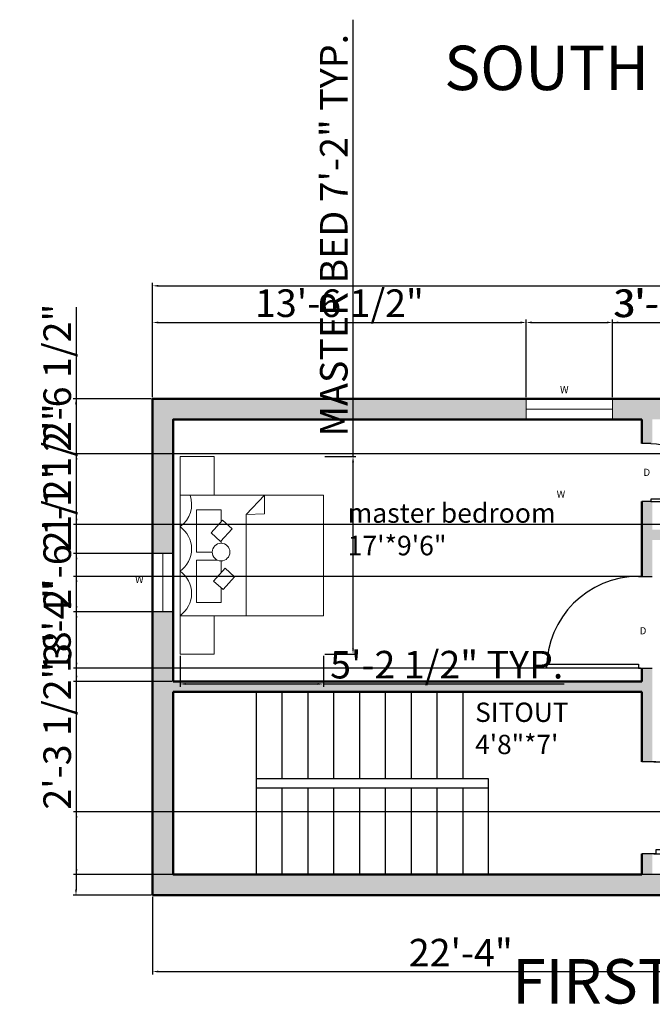
# Model space of a CAD drawing. Units: inches. Extents: x 2225 to 3094, y 1739 to 2599.
# Tile 2 of 5: x 2225 to 2500, y 2171 to 2599. Entities that reach past the tile are written whole.
import ezdxf

# ---------------------------------------------------------------- set-up
doc = ezdxf.new("R2010")
doc.units = ezdxf.units.IN
for name, color, linetype, lineweight in [('A-ANNO-DIMS', 2, 'Continuous', 18), ('A-ANNO-TEXT', 7, 'Continuous', 18), ('A-ANNO-TITL', 7, 'Continuous', 35), ('A-AREA-IDEN', 7, 'Continuous', 18), ('A-DOOR', 4, 'Continuous', 25), ('A-FLOR-STRS', 7, 'Continuous', 25), ('A-FURN', 8, 'Continuous', 18), ('A-WALL-PATT', 160, 'Continuous', 13), ('WALL', 7, 'Continuous', 50), ('WINDOW', 130, 'Continuous', 18)]:
    doc.layers.add(name, color=color, linetype=linetype, lineweight=lineweight)
doc.styles.get("Standard").update_dxf_attribs({"font": 'arial.ttf'})
doc.dimstyles.new('ISO-25', dxfattribs={"dimtxt": 12, "dimasz": 2.5, "dimexe": 1.25, "dimexo": 0.625, "dimtad": 1, "dimdec": 0, "dimlunit": 4, "dimtxsty": 'Standard', "dimcen": 2.5, "dimadec": 0, "dimazin": 0, "dimtfac": 1, "dimtdec": 0, "dimtmove": 0, "dimatfit": 3, "dimfxl": 1, "dimarcsym": 0})

# ---------------------------------------------------------------- blocks, each defined once
blk = doc.blocks.new('*U4')
for p, q in [((0, 0), (0, -6)), ((40, 0), (40, -6))]:
    blk.add_line(p, q)
blk.add_lwpolyline([(0, 0), (0, 40), (1.75, 40), (1.75, 0)], close=True)
blk.add_arc((0, 0), 40, 0, 90)
blk = doc.blocks.new('*D5')
at = {"layer": 'A-ANNO-DIMS', "color": 0, "lineweight": -2, "transparency": 16777216}
for p, q in [((2282.56, 2434.95), (2282.56, 2484.67)), ((2906.56, 2434.95), (2906.56, 2484.67)), ((2285.06, 2483.42), (2904.06, 2483.42))]:
    blk.add_line(p, q, dxfattribs=at)
at = {"layer": 'A-ANNO-DIMS', "color": 0, "transparency": 16777216}
for points in [[(2285.06, 2483.83), (2285.06, 2483), (2282.56, 2483.42)], [(2904.06, 2483.83), (2904.06, 2483), (2906.56, 2483.42)]]:
    blk.add_solid(points, dxfattribs=at)
at = {"layer": 'Defpoints', "color": 0, "transparency": 16777216}
for p in [(2906.56, 2483.42), (2282.56, 2434.33), (2906.56, 2434.33)]:
    blk.add_point(p, dxfattribs=at)
at = {"layer": 'A-ANNO-DIMS', "color": 0, "transparency": 16777216, "insert": (2594.56, 2490.17), "char_height": 12, "attachment_point": 5}
blk.add_mtext("52'", dxfattribs=at)
blk = doc.blocks.new('*D6')
at = {"layer": 'A-ANNO-DIMS', "color": 0, "lineweight": -2, "transparency": 16777216}
for p, q in [((2281.93, 2434.33), (2247.95, 2434.33)), ((2249.2, 2431.83), (2249.2, 2220.83)), ((2281.93, 2218.33), (2247.95, 2218.33))]:
    blk.add_line(p, q, dxfattribs=at)
at = {"layer": 'A-ANNO-DIMS', "color": 0, "transparency": 16777216}
for points in [[(2248.78, 2431.83), (2249.61, 2431.83), (2249.2, 2434.33)], [(2248.78, 2220.83), (2249.61, 2220.83), (2249.2, 2218.33)]]:
    blk.add_solid(points, dxfattribs=at)
at = {"layer": 'Defpoints', "color": 0, "transparency": 16777216}
for p in [(2282.56, 2434.33), (2249.2, 2218.33), (2282.56, 2218.33)]:
    blk.add_point(p, dxfattribs=at)
at = {"layer": 'A-ANNO-DIMS', "color": 0, "transparency": 16777216, "insert": (2242.45, 2326.33), "char_height": 12, "attachment_point": 5, "rotation": 90}
blk.add_mtext("18'", dxfattribs=at)
blk = doc.blocks.new('STAIR-RETURN')
for p, q in [((0, 79.5), (36, 79.5)), ((36, 79.5), (36, 0)), ((47.27, 79.5), (47.27, 41.75)), ((58.52, 79.5), (58.52, 41.75)), ((69.77, 79.5), (69.77, 41.75)), ((81.01, 79.5), (81.01, 41.75)), ((92.26, 79.5), (92.26, 41.75)), ((103.51, 79.5), (103.51, 41.75)), ((114.75, 79.5), (114.75, 41.75)), ((204, 79.5), (126, 79.5)), ((126, 79.5), (126, 41.75)), ((36, 41.75), (126, 41.75)), ((126, 41.75), (137, 41.75)), ((137, 41.75), (137, 0)), ((36, 37.75), (126, 37.75)), ((47.27, 37.75), (47.27, 0)), ((58.52, 37.75), (58.52, 0)), ((69.77, 37.75), (69.77, 0)), ((81.01, 37.75), (81.01, 0)), ((92.26, 37.75), (92.26, 0)), ((103.51, 37.75), (103.51, 0)), ((114.75, 37.75), (114.75, 0)), ((126, 37.75), (137, 37.75)), ((126, 37.75), (126, 0))]:
    blk.add_line(p, q)
blk = doc.blocks.new('BED-MASTER')
for p, q in [((28.8, 60.76), (36.78, 69.23)), ((36.78, 69.23), (36.78, 61.09)), ((36.78, 61.09), (28.8, 60.76)), ((28.8, 16.79), (28.8, 60.76))]:
    blk.add_line(p, q)
for points in [[(0, 69.23), (14.9, 69.23), (14.9, 86.02), (0, 86.02)], [(0, 16.79), (62.39, 16.79), (62.39, 69.23), (0, 69.23)], [(13.53, 52.86), (18.54, 58.39), (22.68, 54.63), (17.67, 49.11)], [(14.58, 31.86), (19.59, 37.39), (23.73, 33.63), (18.72, 28.11)], [(0, 0), (14.9, 0), (14.9, 16.79), (0, 16.79)]]:
    blk.add_lwpolyline(points, close=True)
for points in [[(17.87, 57.65), (17.87, 62.86), (7.1, 62.86), (7.1, 44.44), (14.04, 44.44)], [(17.87, 48.27), (17.87, 49.33)], [(16.36, 40.92), (7.1, 40.92), (7.1, 22.51), (17.87, 22.51), (17.87, 28.87)], [(17.87, 35.5), (17.87, 40.61)]]:
    blk.add_lwpolyline(points)
blk.add_circle((17.87, 44.44), 3.83)
for centre, end in [((-6.76, 65.2), 19.9878), ((-6.76, 45.83), 55.0719), ((-6.76, 26.47), 55.0719)]:
    blk.add_arc(centre, 11.81, 304.9281, end)
blk = doc.blocks.new('*D24')
at = {"layer": 'A-ANNO-DIMS', "color": 0, "lineweight": -2, "transparency": 16777216}
for p, q in [((2369.78, 2409.18), (2369.78, 2599.17)), ((2357.5, 2409.18), (2371.03, 2409.18)), ((2369.78, 2325.67), (2369.78, 2406.68)), ((2357.5, 2323.17), (2371.03, 2323.17))]:
    blk.add_line(p, q, dxfattribs=at)
at = {"layer": 'A-ANNO-DIMS', "color": 0, "transparency": 16777216}
for points in [[(2369.36, 2406.68), (2370.2, 2406.68), (2369.78, 2409.18)], [(2369.36, 2325.67), (2370.2, 2325.67), (2369.78, 2323.17)]]:
    blk.add_solid(points, dxfattribs=at)
at = {"layer": 'Defpoints', "color": 0, "transparency": 16777216}
for p in [(2356.88, 2409.18), (2369.78, 2409.18), (2356.88, 2323.17)]:
    blk.add_point(p, dxfattribs=at)
at = {"layer": 'A-ANNO-DIMS', "color": 0, "transparency": 16777216, "insert": (2362.95, 2505.43), "char_height": 12, "attachment_point": 5, "rotation": 90}
blk.add_mtext('MASTER BED 7\'-2" TYP.', dxfattribs=at)
blk = doc.blocks.new('*D25')
at = {"layer": 'A-ANNO-DIMS', "color": 0, "lineweight": -2, "transparency": 16777216}
for p, q in [((2294.48, 2322.54), (2294.48, 2309.01)), ((2356.88, 2322.54), (2356.88, 2309.01)), ((2296.98, 2310.26), (2354.38, 2310.26)), ((2356.88, 2310.26), (2461.73, 2310.26))]:
    blk.add_line(p, q, dxfattribs=at)
at = {"layer": 'A-ANNO-DIMS', "color": 0, "transparency": 16777216}
for points in [[(2296.98, 2310.68), (2296.98, 2309.85), (2294.48, 2310.26)], [(2354.38, 2310.68), (2354.38, 2309.85), (2356.88, 2310.26)]]:
    blk.add_solid(points, dxfattribs=at)
at = {"layer": 'Defpoints', "color": 0, "transparency": 16777216}
for p in [(2294.48, 2323.17), (2356.88, 2323.17), (2356.88, 2310.26)]:
    blk.add_point(p, dxfattribs=at)
at = {"layer": 'A-ANNO-DIMS', "color": 0, "transparency": 16777216, "insert": (2410.56, 2317.09), "char_height": 12, "attachment_point": 5}
blk.add_mtext('5\'-2 1/2" TYP.', dxfattribs=at)
blk = doc.blocks.new('*D54')
at = {"layer": 'A-ANNO-DIMS', "color": 0, "lineweight": -2, "transparency": 16777216}
for p, q in [((2282.56, 2434.95), (2282.56, 2468.73)), ((2285.06, 2467.48), (2442.66, 2467.48)), ((2445.16, 2434.95), (2445.16, 2468.73))]:
    blk.add_line(p, q, dxfattribs=at)
at = {"layer": 'A-ANNO-DIMS', "color": 0, "transparency": 16777216}
for points in [[(2285.06, 2467.89), (2285.06, 2467.06), (2282.56, 2467.48)], [(2442.66, 2467.89), (2442.66, 2467.06), (2445.16, 2467.48)]]:
    blk.add_solid(points, dxfattribs=at)
at = {"layer": 'Defpoints', "color": 0, "transparency": 16777216}
for p in [(2445.16, 2467.48), (2282.56, 2434.33), (2445.16, 2434.33)]:
    blk.add_point(p, dxfattribs=at)
at = {"layer": 'A-ANNO-DIMS', "color": 0, "transparency": 16777216, "insert": (2363.86, 2474.31), "char_height": 12, "attachment_point": 5}
blk.add_mtext('13\'-6 1/2"', dxfattribs=at)
blk = doc.blocks.new('*D55')
at = {"layer": 'A-ANNO-DIMS', "color": 0, "lineweight": -2, "transparency": 16777216}
for p, q in [((2445.16, 2434.95), (2445.16, 2468.73)), ((2447.66, 2467.48), (2480.26, 2467.48)), ((2482.76, 2434.95), (2482.76, 2468.73)), ((2482.76, 2467.48), (2546.36, 2467.48))]:
    blk.add_line(p, q, dxfattribs=at)
at = {"layer": 'A-ANNO-DIMS', "color": 0, "transparency": 16777216}
for points in [[(2447.66, 2467.89), (2447.66, 2467.06), (2445.16, 2467.48)], [(2480.26, 2467.89), (2480.26, 2467.06), (2482.76, 2467.48)]]:
    blk.add_solid(points, dxfattribs=at)
at = {"layer": 'Defpoints', "color": 0, "transparency": 16777216}
for p in [(2482.76, 2467.48), (2445.16, 2434.33), (2482.76, 2434.33)]:
    blk.add_point(p, dxfattribs=at)
at = {"layer": 'A-ANNO-DIMS', "color": 0, "transparency": 16777216, "insert": (2515.81, 2474.31), "char_height": 12, "attachment_point": 5}
blk.add_mtext('3\'-1 1/2"', dxfattribs=at)
blk = doc.blocks.new('*D56')
at = {"layer": 'A-ANNO-DIMS', "color": 0, "lineweight": -2, "transparency": 16777216}
for p, q in [((2482.76, 2434.95), (2482.76, 2468.73)), ((2485.26, 2467.48), (2526.19, 2467.48)), ((2528.69, 2434.95), (2528.69, 2468.73))]:
    blk.add_line(p, q, dxfattribs=at)
at = {"layer": 'A-ANNO-DIMS', "color": 0, "transparency": 16777216}
for points in [[(2485.26, 2467.89), (2485.26, 2467.06), (2482.76, 2467.48)], [(2526.19, 2467.89), (2526.19, 2467.06), (2528.69, 2467.48)]]:
    blk.add_solid(points, dxfattribs=at)
at = {"layer": 'Defpoints', "color": 0, "transparency": 16777216}
for p in [(2528.69, 2467.48), (2482.76, 2434.33), (2528.69, 2434.33)]:
    blk.add_point(p, dxfattribs=at)
at = {"layer": 'A-ANNO-DIMS', "color": 0, "transparency": 16777216, "insert": (2505.72, 2474.23), "char_height": 12, "attachment_point": 5}
blk.add_mtext('3\'-10"', dxfattribs=at)
blk = doc.blocks.new('*D63')
at = {"layer": 'A-ANNO-DIMS', "color": 0, "lineweight": -2, "transparency": 16777216}
for p, q in [((2249.41, 2341.62), (2249.41, 2405.44)), ((2290.93, 2341.62), (2248.16, 2341.62)), ((2249.41, 2313.83), (2249.41, 2339.12)), ((2290.93, 2311.33), (2248.16, 2311.33))]:
    blk.add_line(p, q, dxfattribs=at)
at = {"layer": 'A-ANNO-DIMS', "color": 0, "transparency": 16777216}
for points in [[(2248.99, 2339.12), (2249.82, 2339.12), (2249.41, 2341.62)], [(2248.99, 2313.83), (2249.82, 2313.83), (2249.41, 2311.33)]]:
    blk.add_solid(points, dxfattribs=at)
at = {"layer": 'Defpoints', "color": 0, "transparency": 16777216}
for p in [(2249.41, 2341.62), (2291.56, 2341.62), (2291.56, 2311.33)]:
    blk.add_point(p, dxfattribs=at)
at = {"layer": 'A-ANNO-DIMS', "color": 0, "transparency": 16777216, "insert": (2242.58, 2374.78), "char_height": 12, "attachment_point": 5, "rotation": 90}
blk.add_mtext('2\'-6 1/2"', dxfattribs=at)
blk = doc.blocks.new('*D64')
at = {"layer": 'A-ANNO-DIMS', "color": 0, "lineweight": -2, "transparency": 16777216}
for p, q in [((2249.41, 2366.97), (2249.41, 2430.79)), ((2290.93, 2366.97), (2248.16, 2366.97)), ((2249.41, 2344.12), (2249.41, 2364.47)), ((2290.93, 2341.62), (2248.16, 2341.62))]:
    blk.add_line(p, q, dxfattribs=at)
at = {"layer": 'A-ANNO-DIMS', "color": 0, "transparency": 16777216}
for points in [[(2248.99, 2364.47), (2249.82, 2364.47), (2249.41, 2366.97)], [(2248.99, 2344.12), (2249.82, 2344.12), (2249.41, 2341.62)]]:
    blk.add_solid(points, dxfattribs=at)
at = {"layer": 'Defpoints', "color": 0, "transparency": 16777216}
for p in [(2249.41, 2366.97), (2291.56, 2366.97), (2291.56, 2341.62)]:
    blk.add_point(p, dxfattribs=at)
at = {"layer": 'A-ANNO-DIMS', "color": 0, "transparency": 16777216, "insert": (2242.58, 2400.13), "char_height": 12, "attachment_point": 5, "rotation": 90}
blk.add_mtext('2\'-1 1/2"', dxfattribs=at)
blk = doc.blocks.new('*D66')
at = {"layer": 'A-ANNO-DIMS', "color": 0, "lineweight": -2, "transparency": 16777216}
for p, q in [((2282.56, 2217.7), (2282.56, 2183.93)), ((2550.8, 2217.7), (2550.8, 2183.93)), ((2285.06, 2185.18), (2548.3, 2185.18))]:
    blk.add_line(p, q, dxfattribs=at)
at = {"layer": 'A-ANNO-DIMS', "color": 0, "transparency": 16777216}
for points in [[(2285.06, 2185.59), (2285.06, 2184.76), (2282.56, 2185.18)], [(2548.3, 2185.59), (2548.3, 2184.76), (2550.8, 2185.18)]]:
    blk.add_solid(points, dxfattribs=at)
at = {"layer": 'Defpoints', "color": 0, "transparency": 16777216}
for p in [(2282.56, 2218.33), (2550.8, 2218.33), (2550.8, 2185.18)]:
    blk.add_point(p, dxfattribs=at)
at = {"layer": 'A-ANNO-DIMS', "color": 0, "transparency": 16777216, "insert": (2416.68, 2191.83), "char_height": 12, "attachment_point": 5}
blk.add_mtext('22\'-4"', dxfattribs=at)
blk = doc.blocks.new('*D68')
at = {"layer": 'A-ANNO-DIMS', "color": 0, "lineweight": -2, "transparency": 16777216}
for p, q in [((2500.68, 2276.4), (2940.96, 2276.4)), ((2939.71, 2273.9), (2939.71, 2238.9)), ((2500.68, 2236.4), (2940.96, 2236.4))]:
    blk.add_line(p, q, dxfattribs=at)
at = {"layer": 'A-ANNO-DIMS', "color": 0, "transparency": 16777216}
for points in [[(2939.29, 2273.9), (2940.12, 2273.9), (2939.71, 2276.4)], [(2939.29, 2238.9), (2940.12, 2238.9), (2939.71, 2236.4)]]:
    blk.add_solid(points, dxfattribs=at)
at = {"layer": 'Defpoints', "color": 0, "transparency": 16777216}
for p in [(2500.06, 2276.4), (2500.06, 2236.4), (2939.71, 2236.4)]:
    blk.add_point(p, dxfattribs=at)
at = {"layer": 'A-ANNO-DIMS', "color": 0, "transparency": 16777216, "insert": (2932.95, 2256.4), "char_height": 12, "attachment_point": 5, "rotation": 90}
blk.add_mtext('3\'-4"', dxfattribs=at)
blk = doc.blocks.new('*D69')
at = {"layer": 'A-ANNO-DIMS', "color": 0, "lineweight": -2, "transparency": 16777216}
for p, q in [((2494.93, 2357.06), (2248.16, 2357.06)), ((2249.41, 2319.56), (2249.41, 2354.56)), ((2494.93, 2317.06), (2248.16, 2317.06))]:
    blk.add_line(p, q, dxfattribs=at)
at = {"layer": 'A-ANNO-DIMS', "color": 0, "transparency": 16777216}
for points in [[(2248.99, 2354.56), (2249.82, 2354.56), (2249.41, 2357.06)], [(2248.99, 2319.56), (2249.82, 2319.56), (2249.41, 2317.06)]]:
    blk.add_solid(points, dxfattribs=at)
at = {"layer": 'Defpoints', "color": 0, "transparency": 16777216}
for p in [(2249.41, 2357.06), (2495.56, 2357.06), (2495.56, 2317.06)]:
    blk.add_point(p, dxfattribs=at)
at = {"layer": 'A-ANNO-DIMS', "color": 0, "transparency": 16777216, "insert": (2242.65, 2337.06), "char_height": 12, "attachment_point": 5, "rotation": 90}
blk.add_mtext('3\'-4"', dxfattribs=at)
blk = doc.blocks.new('*D72')
at = {"layer": 'A-ANNO-DIMS', "color": 0, "lineweight": -2, "transparency": 16777216}
for p, q in [((2249.41, 2410.28), (2249.41, 2474.1)), ((2653.84, 2410.28), (2248.16, 2410.28)), ((2249.41, 2382.17), (2249.41, 2407.78)), ((2653.84, 2379.67), (2248.16, 2379.67))]:
    blk.add_line(p, q, dxfattribs=at)
at = {"layer": 'A-ANNO-DIMS', "color": 0, "transparency": 16777216}
for points in [[(2248.99, 2407.78), (2249.82, 2407.78), (2249.41, 2410.28)], [(2248.99, 2382.17), (2249.82, 2382.17), (2249.41, 2379.67)]]:
    blk.add_solid(points, dxfattribs=at)
at = {"layer": 'Defpoints', "color": 0, "transparency": 16777216}
for p in [(2249.41, 2410.28), (2654.47, 2410.28), (2654.47, 2379.67)]:
    blk.add_point(p, dxfattribs=at)
at = {"layer": 'A-ANNO-DIMS', "color": 0, "transparency": 16777216, "insert": (2242.58, 2443.44), "char_height": 12, "attachment_point": 5, "rotation": 90}
blk.add_mtext('2\'-6 1/2"', dxfattribs=at)
blk = doc.blocks.new('*D75')
at = {"layer": 'A-ANNO-DIMS', "color": 0, "lineweight": -2, "transparency": 16777216}
for p, q in [((2249.41, 2254.61), (2249.41, 2318.43)), ((2727.01, 2254.61), (2248.16, 2254.61)), ((2249.41, 2229.83), (2249.41, 2252.11)), ((2727.01, 2227.33), (2248.16, 2227.33))]:
    blk.add_line(p, q, dxfattribs=at)
at = {"layer": 'A-ANNO-DIMS', "color": 0, "transparency": 16777216}
for points in [[(2248.99, 2252.11), (2249.82, 2252.11), (2249.41, 2254.61)], [(2248.99, 2229.83), (2249.82, 2229.83), (2249.41, 2227.33)]]:
    blk.add_solid(points, dxfattribs=at)
at = {"layer": 'Defpoints', "color": 0, "transparency": 16777216}
for p in [(2249.41, 2254.61), (2727.64, 2254.61), (2727.64, 2227.33)]:
    blk.add_point(p, dxfattribs=at)
at = {"layer": 'A-ANNO-DIMS', "color": 0, "transparency": 16777216, "insert": (2242.57, 2287.77), "char_height": 12, "attachment_point": 5, "rotation": 90}
blk.add_mtext('2\'-3 1/2"', dxfattribs=at)

msp = doc.modelspace()

# ---------------------------------------------------------------- hatches: boundary and pattern name
at = {"layer": 'A-WALL-PATT'}
h = msp.add_hatch(color=256, dxfattribs=at)
h.dxf.hatch_style = 1
h.paths.add_polyline_path([(2445.16, 2434.33), (2282.56, 2434.33), (2282.56, 2366.97), (2291.56, 2366.97), (2291.56, 2425.33), (2445.16, 2425.33)], flags=17)
h.paths.add_polyline_path([(2528.69, 2434.33), (2482.76, 2434.33), (2482.76, 2425.33), (2495.56, 2425.33), (2495.56, 2414.78), (2499.34, 2414.78, -0.007163), (2500.06, 2414.76), (2500.06, 2425.33), (2528.69, 2425.33)], flags=17)
h.paths.add_polyline_path([(2867.81, 2330.83), (2783.56, 2330.83), (2783.56, 2354.83), (2783.56, 2425.33), (2801.54, 2425.33), (2801.54, 2434.33), (2758.39, 2434.33), (2758.39, 2425.33), (2779.06, 2425.33), (2779.06, 2330.83), (2767.43, 2330.83), (2767.43, 2326.33), (2779.06, 2326.33), (2779.06, 2307.37), (2783.56, 2307.37), (2783.56, 2326.33), (2867.81, 2326.33)])
h.paths.add_polyline_path([(2906.56, 2434.33), (2839.14, 2434.33), (2839.14, 2425.33), (2897.56, 2425.33), (2897.56, 2330.83), (2897.56, 2326.33), (2897.56, 2264.13), (2906.56, 2264.13)])
h.paths.add_polyline_path([(2906.56, 2236.32), (2897.56, 2236.32), (2897.56, 2227.33), (2860.08, 2227.33), (2860.08, 2218.33), (2906.56, 2218.33)])
h.paths.add_polyline_path([(2815.14, 2227.33), (2783.56, 2227.33), (2779.06, 2227.33), (2727.64, 2227.33), (2606.48, 2227.33), (2606.48, 2218.33), (2815.14, 2218.33)])
h.paths.add_polyline_path([(2780.45, 2273.09), (2785.35, 2273.09), (2785.35, 2279.46), (2780.45, 2279.46)], flags=9)
h.paths.add_polyline_path([(2500.16, 2250.57), (2508.42, 2250.57), (2508.42, 2256.93), (2500.16, 2256.93)], flags=25)
h.paths.add_polyline_path([(2745.49, 2326.59), (2750.15, 2326.59), (2750.15, 2332.96), (2745.49, 2332.96)], flags=9)
h.paths.add_polyline_path([(2651.86, 2391.09), (2656.53, 2391.09), (2656.53, 2397.46), (2651.86, 2397.46)], flags=9)
h.paths.add_polyline_path([(2493.47, 2330.16), (2498.13, 2330.16), (2498.13, 2336.53), (2493.47, 2336.53)], flags=25)
h.paths.add_polyline_path([(2530.27, 2348.62), (2534.93, 2348.62), (2534.93, 2354.99), (2530.27, 2354.99)], flags=25)
h.paths.add_polyline_path([(2432.89, 2282.56), (2450.26, 2282.56), (2450.26, 2294.09), (2432.89, 2294.09)], flags=25)
h.paths.add_polyline_path([(2735.79, 2240.68), (2748.37, 2240.68), (2748.37, 2247.05), (2735.79, 2247.05)], flags=9)
h.paths.add_polyline_path([(2717.02, 2288.94), (2747.35, 2288.94), (2747.35, 2300.47), (2717.02, 2300.47)], flags=9)
h.paths.add_polyline_path([(2839.5, 2270.61), (2856.29, 2270.61), (2856.29, 2282.14), (2839.5, 2282.14)], flags=25)
h.paths.add_polyline_path([(2825.64, 2385.51), (2846.28, 2385.51), (2846.28, 2397.04), (2825.64, 2397.04)], flags=25)
h.paths.add_polyline_path([(2692.05, 2396.34), (2722.05, 2396.34), (2722.05, 2407.87), (2692.05, 2407.87)], flags=9)
h.paths.add_polyline_path([(2282.56, 2366.97), (2291.56, 2366.97), (2291.56, 2425.33), (2445.16, 2425.33), (2445.16, 2434.33), (2282.56, 2434.33)])
h.paths.add_polyline_path([(2291.56, 2341.62), (2282.56, 2341.62), (2282.56, 2218.33), (2550.8, 2218.33), (2550.8, 2227.33), (2500.06, 2227.33), (2500.06, 2236.4), (2495.56, 2236.4), (2495.56, 2227.33), (2291.56, 2227.33), (2291.56, 2306.83), (2327.56, 2306.83), (2495.56, 2306.83), (2495.56, 2276.4), (2500.06, 2276.4), (2500.06, 2306.83), (2500.06, 2317.06), (2495.56, 2317.06), (2495.56, 2311.33), (2291.56, 2311.33)])
h = msp.add_hatch(color=256, dxfattribs=at)
h.dxf.hatch_style = 1
h.paths.add_polyline_path([(2727.43, 2330.83), (2659.06, 2330.83), (2659.06, 2379.67), (2654.56, 2379.67), (2654.56, 2377.33), (2582.56, 2377.33), (2582.56, 2425.33), (2603.88, 2425.33), (2603.88, 2434.33), (2552.55, 2434.33), (2552.55, 2425.33), (2578.06, 2425.33), (2578.06, 2377.33), (2500.06, 2377.33), (2500.06, 2389.59), (2499.34, 2389.59), (2495.56, 2389.59), (2495.56, 2357.06), (2500.06, 2357.06), (2500.06, 2372.83), (2530.06, 2372.83), (2530.06, 2364.02), (2533.84, 2364.02, -0.007163), (2534.56, 2364.01), (2534.56, 2372.83), (2578.06, 2372.83), (2582.56, 2372.83), (2654.56, 2372.83), (2654.56, 2330.83), (2582.56, 2330.83), (2581.71, 2330.83), (2578.06, 2330.83), (2534.56, 2330.83), (2534.56, 2338.83), (2533.84, 2338.83), (2530.06, 2338.83), (2530.06, 2326.33), (2659.06, 2326.33), (2727.43, 2326.33)])
h.paths.add_polyline_path([(2720.79, 2434.33), (2627.74, 2434.33), (2627.74, 2425.33), (2654.56, 2425.33), (2654.56, 2410.28), (2659.06, 2410.28), (2659.06, 2425.33), (2720.79, 2425.33)], flags=17)
h.paths.add_polyline_path([(2445.16, 2434.33), (2282.56, 2434.33), (2282.56, 2366.97), (2291.56, 2366.97), (2291.56, 2425.33), (2445.16, 2425.33)])

# ---------------------------------------------------------------- linework, layer by layer
at = {"layer": 'WALL'}
for p, q in [((2291.56, 2425.33), (2495.56, 2425.33)), ((2495.56, 2425.33), (2495.56, 2414.78)), ((2495.56, 2389.59), (2495.56, 2357.06)), ((2495.56, 2317.06), (2495.56, 2311.33)), ((2495.56, 2311.33), (2291.56, 2311.33)), ((2495.56, 2306.83), (2291.56, 2306.83)), ((2495.56, 2306.83), (2495.56, 2276.4)), ((2495.56, 2236.4), (2495.56, 2227.33))]:
    msp.add_line(p, q, dxfattribs=at)
msp.add_lwpolyline([(2282.56, 2218.33), (2906.56, 2218.33), (2906.56, 2434.33), (2282.56, 2434.33)], close=True, dxfattribs=at)
for points in [[(2495.56, 2425.33), (2291.56, 2425.33), (2291.56, 2311.33)], [(2291.56, 2306.83), (2291.56, 2227.33), (2495.56, 2227.33)]]:
    msp.add_lwpolyline(points, dxfattribs=at)
at = {"layer": 'WINDOW'}
for p, q in [((2445.16, 2429.83), (2482.76, 2429.83)), ((2287.06, 2366.97), (2287.06, 2341.62))]:
    msp.add_line(p, q, dxfattribs=at)
for points in [[(2482.76, 2425.33), (2445.16, 2425.33), (2445.16, 2434.33), (2482.76, 2434.33)], [(2282.56, 2366.97), (2291.56, 2366.97), (2291.56, 2341.62), (2282.56, 2341.62)]]:
    msp.add_lwpolyline(points, close=True, dxfattribs=at)

# ---------------------------------------------------------------- block references
at = {"layer": 'A-DOOR', "xscale": -0.6297308224195742, "yscale": 0.6297308224195742, "zscale": 0.6297308224195742, "rotation": 270}
msp.add_blockref('*U4', (2499.34, 2389.59), dxfattribs=at)
at = {"layer": 'A-DOOR', "rotation": 89.99999999999999}
msp.add_blockref('*U4', (2494.06, 2317.06), dxfattribs=at)
at = {"layer": 'A-DOOR', "xscale": -1, "rotation": 270}
msp.add_blockref('*U4', (2501.56, 2236.4), dxfattribs=at)
at = {"layer": 'A-FLOR-STRS'}
msp.add_blockref('STAIR-RETURN', (2291.56, 2227.33), dxfattribs=at)
at = {"layer": 'A-FURN'}
msp.add_blockref('BED-MASTER', (2294.48, 2323.17), dxfattribs=at)

# ---------------------------------------------------------------- texts
at = {"layer": 'A-ANNO-TEXT', "char_height": 3.09, "attachment_point": 1}
for s, insert in [('W', (2459.89, 2439.82)), ('D', (2496.21, 2403.86)), ('W', (2458.43, 2394.32)), ('W', (2274.93, 2357.26)), ('D', (2494.57, 2334.94))]:
    msp.add_mtext_dynamic_manual_height_columns(s, width=49.525, gutter_width=15.45, heights=[0], dxfattribs=dict(at, insert=insert))
at = {"layer": 'A-ANNO-TITL', "char_height": 19.3093, "attachment_point": 1}
for s, insert in [('SOUTH FACING HOUSE PLAN', (2409.47, 2587.86)), ('FIRST FLOOR HOUSE PLAN', (2439.06, 2190.58))]:
    msp.add_mtext_dynamic_manual_height_columns(s, width=2944.6637, gutter_width=96.55, heights=[0], dxfattribs=dict(at, insert=insert))
at = {"layer": 'A-AREA-IDEN', "attachment_point": 1}
for s, width, gutter_width, insert, char_height in [('master bedroom\\P17\'*9\'6"', 136.0341, 42.44, (2367.43, 2388.85), 8.4873), ('SITOUT\\P4\'8"*7\'', 134.5511, 41.97, (2422.94, 2302.14), 8.395)]:
    msp.add_mtext_dynamic_manual_height_columns(s, width=width, gutter_width=gutter_width, heights=[0], dxfattribs=dict(at, insert=insert, char_height=char_height))

# ---------------------------------------------------------------- dimensions: what is measured, and where the dimension line sits
at = {"layer": 'A-ANNO-DIMS'}
dim = msp.add_linear_dim(base=(2369.78, 2409.18), p1=(2356.88, 2323.17), p2=(2356.88, 2409.18), angle=90, text='MASTER BED <> TYP.', dimstyle='ISO-25', override={"dimdec": 1, "dimlfac": 1, "dimrnd": 0, "dimzin": 1, "dimdsep": 46, "dimlunit": 4, "dimfrac": 2}, dxfattribs=at)
dim.commit()
dim.dimension.update_dxf_attribs({"geometry": '*D24', "text_midpoint": (2362.95, 2505.43)})
for base, p1, p2, override, picture, middle in [((2906.56, 2483.42), (2282.56, 2434.33), (2906.56, 2434.33), {"dimclrd": 0, "dimclre": 0, "dimclrt": 0}, '*D5', (2594.56, 2490.17)), ((2445.16, 2467.48), (2282.56, 2434.33), (2445.16, 2434.33), {"dimdec": 1, "dimlfac": 1, "dimrnd": 0, "dimzin": 1, "dimdsep": 46, "dimlunit": 4, "dimfrac": 2}, '*D54', (2363.86, 2474.31)), ((2482.76, 2467.48), (2445.16, 2434.33), (2482.76, 2434.33), {"dimdec": 1, "dimlfac": 1, "dimrnd": 0, "dimzin": 1, "dimdsep": 46, "dimlunit": 4, "dimfrac": 2}, '*D55', (2515.81, 2474.31)), ((2528.69, 2467.48), (2482.76, 2434.33), (2528.69, 2434.33), {"dimdec": 1, "dimlfac": 1, "dimrnd": 0, "dimzin": 1, "dimdsep": 46, "dimlunit": 4, "dimfrac": 2}, '*D56', (2505.72, 2474.23)), ((2550.8, 2185.18), (2282.56, 2218.33), (2550.8, 2218.33), {"dimdec": 1, "dimlfac": 1, "dimrnd": 0, "dimzin": 1, "dimdsep": 46, "dimlunit": 4, "dimfrac": 2}, '*D66', (2416.68, 2191.83))]:
    dim = msp.add_linear_dim(base=base, p1=p1, p2=p2, dimstyle='ISO-25', override=override, dxfattribs=at)
    dim.commit()
    dim.dimension.update_dxf_attribs({"geometry": picture, "text_midpoint": middle})
for base, p1, p2, override, picture, middle in [((2249.41, 2410.28), (2654.47, 2379.67), (2654.47, 2410.28), {"dimdec": 1, "dimlfac": 1, "dimrnd": 0, "dimzin": 1, "dimdsep": 46, "dimlunit": 4, "dimfrac": 2}, '*D72', (2242.58, 2443.44)), ((2249.2, 2218.33), (2282.56, 2434.33), (2282.56, 2218.33), {"dimclrd": 0, "dimclre": 0, "dimclrt": 0}, '*D6', (2242.45, 2326.33)), ((2249.4075, 2366.9723), (2291.5575, 2341.6221), (2291.5575, 2366.9723), {"dimdec": 1, "dimlfac": 1, "dimrnd": 0, "dimzin": 1, "dimdsep": 46, "dimlunit": 4, "dimfrac": 2}, '*D64', (2242.5779, 2400.1301)), ((2249.41, 2341.62), (2291.56, 2311.33), (2291.56, 2341.62), {"dimdec": 1, "dimlfac": 1, "dimrnd": 0, "dimzin": 1, "dimdsep": 46, "dimlunit": 4, "dimfrac": 2}, '*D63', (2242.58, 2374.78)), ((2249.41, 2357.06), (2495.56, 2317.06), (2495.56, 2357.06), {"dimdec": 1, "dimlfac": 1, "dimrnd": 0, "dimzin": 1, "dimdsep": 46, "dimlunit": 4, "dimfrac": 2}, '*D69', (2242.65, 2337.06)), ((2249.41, 2254.61), (2727.64, 2227.33), (2727.64, 2254.61), {"dimdec": 1, "dimlfac": 1, "dimrnd": 0, "dimzin": 1, "dimdsep": 46, "dimlunit": 4, "dimfrac": 2}, '*D75', (2242.57, 2287.77)), ((2939.71, 2236.4), (2500.06, 2276.4), (2500.06, 2236.4), {"dimdec": 1, "dimlfac": 1, "dimrnd": 0, "dimzin": 1, "dimdsep": 46, "dimlunit": 4, "dimfrac": 2}, '*D68', (2932.95, 2256.4))]:
    dim = msp.add_linear_dim(base=base, p1=p1, p2=p2, angle=90, dimstyle='ISO-25', override=override, dxfattribs=at)
    dim.commit()
    dim.dimension.update_dxf_attribs({"geometry": picture, "text_midpoint": middle})
dim = msp.add_linear_dim(base=(2356.88, 2310.26), p1=(2294.48, 2323.17), p2=(2356.88, 2323.17), text='<> TYP.', dimstyle='ISO-25', override={"dimdec": 1, "dimlfac": 1, "dimrnd": 0, "dimzin": 1, "dimdsep": 46, "dimlunit": 4, "dimfrac": 2}, dxfattribs=at)
dim.commit()
dim.dimension.update_dxf_attribs({"geometry": '*D25', "text_midpoint": (2410.56, 2317.09)})

doc.saveas('drawing.dxf')
